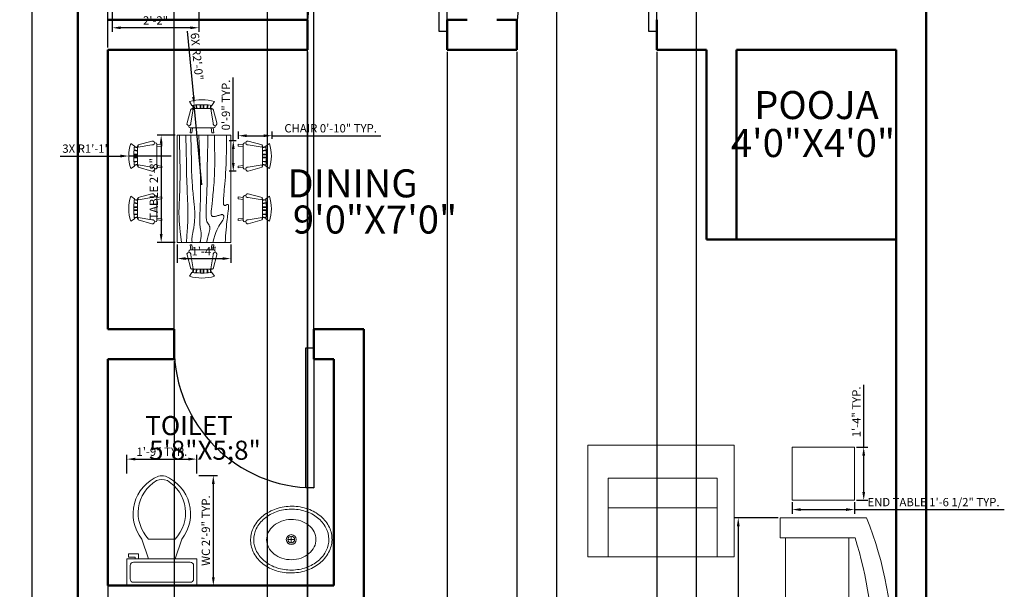
# Model space of a CAD drawing. Units: inches. Extents: x 758743 to 759108, y 3712801 to 3713581.
# Tile 3 of 4: x 758768 to 759064, y 3713244 to 3713415. Entities that reach past the tile are written whole.
import ezdxf

# ---------------------------------------------------------------- set-up
doc = ezdxf.new("R2010")
doc.units = ezdxf.units.IN
for name, color, linetype, lineweight in [('A-ANNO-DIMS', 2, 'Continuous', 18), ('A-AREA-IDEN', 3, 'Continuous', 18), ('A-FLOR-FIXT', 2, 'Continuous', 18), ('A-FURN', 2, 'Continuous', 18), ('DOOR', 4, 'Continuous', 25), ('WALL', 7, 'Continuous', 50)]:
    doc.layers.add(name, color=color, linetype=linetype, lineweight=lineweight)
doc.styles.get("Standard").update_dxf_attribs({"font": 'arial.ttf'})
doc.dimstyles.new('ISO-25', dxfattribs={"dimtxt": 2.5, "dimasz": 2.5, "dimexe": 1.25, "dimexo": 0.625, "dimtad": 1, "dimdec": 0, "dimlunit": 3, "dimtxsty": 'Standard', "dimcen": 2.5, "dimadec": 0, "dimazin": 0, "dimtfac": 1, "dimtdec": 0, "dimtmove": 0, "dimatfit": 3, "dimfxl": 1, "dimarcsym": 0})

# ---------------------------------------------------------------- blocks, each defined once
blk = doc.blocks.new('*U2')
for p, q in [((0, 0), (0, -100)), ((750, 0), (750, -100))]:
    blk.add_line(p, q)
blk.add_lwpolyline([(0, 0), (0, 750), (43.75, 750), (43.75, 0)], close=True)
blk.add_arc((0, 0), 750, 0, 90)
blk = doc.blocks.new('Table - Rectangular Woodgrain 60 x 30 in.')
for p, q in [((0, 0), (0, -30)), ((60, 0), (0, 0)), ((60, -30), (60, 0)), ((0, -30), (60, -30))]:
    blk.add_line(p, q)
for points in [[(0, -2.4), (4.8155, -2.418), (9.0302, -2.4688), (12.709, -2.5477), (15.9167, -2.65), (18.7181, -2.7711), (21.1781, -2.9063), (23.3616, -3.0508), (25.3333, -3.2), (27.1477, -3.3495), (28.8172, -3.4958), (30.3437, -3.636), (31.7291, -3.7667), (32.9756, -3.8849), (34.0849, -3.9875), (35.059, -4.0714), (35.9, -4.1334), (36.6114, -4.1711), (37.2041, -4.1854), (37.6906, -4.1779), (38.0833, -4.15), (38.3948, -4.1034), (38.6375, -4.0396), (38.8239, -3.9602), (38.9666, -3.8667), (39.0764, -3.7608), (39.1573, -3.6448), (39.2116, -3.521), (39.2416, -3.3917), (39.2498, -3.2593), (39.2385, -3.1261), (39.21, -2.9944), (39.1666, -2.8667), (39.111, -2.7447), (39.0468, -2.6281), (38.978, -2.5163), (38.9083, -2.4083), (38.8418, -2.3035), (38.7823, -2.201), (38.7337, -2.1001), (38.7, -2), (38.6844, -1.9003), (38.6875, -1.8021), (38.7094, -1.707), (38.75, -1.6167), (38.8094, -1.5326), (38.8875, -1.4563), (38.9844, -1.3893), (39.1, -1.3333), (39.2351, -1.2896), (39.3937, -1.2583), (39.5804, -1.2396), (39.8, -1.2333), (40.057, -1.2396), (40.3562, -1.2583), (40.7023, -1.2896), (41.1, -1.3333), (41.5547, -1.3895), (42.0755, -1.4573), (42.6721, -1.5361), (43.3542, -1.625), (44.1316, -1.7233), (45.014, -1.8302), (46.0114, -1.9449), (47.1333, -2.0667), (48.3862, -2.1947), (49.7625, -2.3281), (51.2513, -2.4663), (52.8416, -2.6083), (54.5226, -2.7535), (56.2833, -2.9011), (58.1127, -3.0501), (60, -3.2)], [(0, -9.2), (6.5759, -9.0858), (11.9385, -9.0365), (16.2527, -9.0418), (19.6833, -9.0917), (22.3952, -9.1759), (24.5531, -9.2844), (26.322, -9.4069), (27.8666, -9.5333), (29.3241, -9.6553), (30.7203, -9.7719), (32.0532, -9.8837), (33.3208, -9.9917), (34.5213, -10.0965), (35.6526, -10.199), (36.7128, -10.2999), (37.7, -10.4), (38.6129, -10.4996), (39.4531, -10.5969), (40.223, -10.6895), (40.925, -10.775), (41.5613, -10.8512), (42.1344, -10.9156), (42.6465, -10.966), (43.1, -11), (43.4976, -11.0158), (43.8437, -11.0136), (44.143, -10.9942), (44.4, -10.9583), (44.6195, -10.9069), (44.8062, -10.8406), (44.9648, -10.7603), (45.1, -10.6667), (45.2155, -10.5598), (45.3114, -10.4365), (45.3871, -10.2929), (45.4416, -10.125), (45.4743, -9.929), (45.4844, -9.7011), (45.4709, -9.4371), (45.4333, -9.1333), (45.3716, -8.7883), (45.2896, -8.4104), (45.1919, -8.0107), (45.0833, -7.6), (44.9685, -7.1893), (44.8521, -6.7896), (44.7388, -6.4117), (44.6333, -6.0667), (44.54, -5.7628), (44.4614, -5.4979), (44.4001, -5.2675), (44.3583, -5.0667), (44.3384, -4.8909), (44.3427, -4.7354), (44.3736, -4.5956), (44.4333, -4.4667), (44.5236, -4.3453), (44.6427, -4.2333), (44.7884, -4.1339), (44.9583, -4.05), (45.1501, -3.9849), (45.3614, -3.9417), (45.59, -3.9234), (45.8333, -3.9333), (46.0915, -3.9749), (46.3734, -4.0531), (46.6906, -4.1736), (47.0542, -4.3417), (47.4756, -4.5629), (47.9661, -4.8427), (48.5372, -5.1866), (49.2, -5.6), (49.9676, -6.0844), (50.8594, -6.625), (51.8965, -7.2031), (53.1, -7.8), (54.491, -8.3969), (56.0906, -8.975), (57.9199, -9.5156), (60, -10)], [(0, -12.8), (5.1847, -12.9322), (9.6213, -13.0323), (13.3963, -13.1059), (16.5958, -13.1583), (19.3063, -13.1952), (21.614, -13.2219), (23.6054, -13.2439), (25.3666, -13.2667), (26.9728, -13.2947), (28.4531, -13.3281), (29.8256, -13.3663), (31.1083, -13.4083), (32.3191, -13.4535), (33.476, -13.501), (34.597, -13.5501), (35.7, -13.6), (36.7984, -13.6497), (37.8875, -13.6979), (38.9578, -13.743), (40, -13.7833), (41.0047, -13.8174), (41.9625, -13.8438), (42.864, -13.8607), (43.7, -13.8667), (44.4631, -13.8604), (45.1552, -13.8417), (45.7801, -13.8104), (46.3416, -13.7667), (46.8439, -13.7104), (47.2906, -13.6417), (47.6858, -13.5604), (48.0333, -13.4667), (48.3375, -13.3608), (48.6042, -13.2448), (48.8396, -13.121), (49.05, -12.9917), (49.2417, -12.8593), (49.4208, -12.7261), (49.5937, -12.5944), (49.7667, -12.4667), (49.9452, -12.3451), (50.1323, -12.2313), (50.3303, -12.1268), (50.5416, -12.0333), (50.7686, -11.9524), (51.0135, -11.8854), (51.2788, -11.8341), (51.5666, -11.8), (51.8785, -11.7843), (52.2116, -11.7865), (52.562, -11.8059), (52.926, -11.8417), (53.2998, -11.8931), (53.6795, -11.9594), (54.0614, -12.0397), (54.4416, -12.1333), (54.8223, -12.2401), (55.2293, -12.3625), (55.6942, -12.5037), (56.2489, -12.6667), (56.9251, -12.8547), (57.7545, -13.0708), (58.7689, -13.3182), (60, -13.6)], [(0, -18), (5.124, -17.7273), (9.6609, -17.5057), (13.6705, -17.3303), (17.2125, -17.1958), (20.3467, -17.0973), (23.1328, -17.0297), (25.6307, -16.9878), (27.9, -16.9667), (29.9928, -16.9617), (31.9302, -16.9703), (33.7254, -16.9907), (35.3917, -17.0208), (36.9423, -17.0588), (38.3906, -17.1026), (39.7499, -17.1503), (41.0333, -17.2), (42.2519, -17.2496), (43.4073, -17.2969), (44.4986, -17.3395), (45.525, -17.375), (46.4858, -17.4012), (47.3802, -17.4156), (48.2074, -17.416), (48.9667, -17.4), (49.6583, -17.3662), (50.2872, -17.3167), (50.8595, -17.2547), (51.3812, -17.1833), (51.8584, -17.1057), (52.2971, -17.025), (52.7034, -16.9443), (53.0833, -16.8667), (53.443, -16.7951), (53.789, -16.7313), (54.128, -16.6768), (54.4666, -16.6334), (54.8115, -16.6024), (55.1693, -16.5854), (55.5465, -16.5841), (55.95, -16.6), (56.3828, -16.6337), (56.8346, -16.6823), (57.2915, -16.7418), (57.7396, -16.8084), (58.165, -16.878), (58.5539, -16.9469), (58.8924, -17.0111), (59.1666, -17.0667), (59.3679, -17.1107), (59.5078, -17.1438), (59.6032, -17.1675), (59.6708, -17.1833), (59.7275, -17.193), (59.7901, -17.1979), (59.8753, -17.1998), (60, -17.2)], [(0, -22.4), (8.0098, -22.2501), (14.4094, -22.1011), (19.4168, -21.9535), (23.25, -21.8083), (26.1269, -21.6663), (28.2656, -21.5281), (29.884, -21.3947), (31.2, -21.2667), (32.3967, -21.1448), (33.5172, -21.0292), (34.5697, -20.9198), (35.5625, -20.8167), (36.5037, -20.7198), (37.4015, -20.6292), (38.2642, -20.5448), (39.1, -20.4667), (39.9164, -20.3951), (40.7187, -20.3313), (41.5117, -20.2768), (42.3, -20.2333), (43.0883, -20.2024), (43.8812, -20.1854), (44.6836, -20.1841), (45.5, -20.2), (46.3328, -20.234), (47.1747, -20.2844), (48.0163, -20.3488), (48.8479, -20.425), (49.66, -20.5106), (50.4429, -20.6031), (51.1872, -20.7004), (51.8833, -20.8), (52.5246, -20.8999), (53.1166, -20.9995), (53.6681, -21.0983), (54.1875, -21.1958), (54.6834, -21.2919), (55.1646, -21.3859), (55.6394, -21.4777), (56.1167, -21.5667), (56.6028, -21.6515), (57.0961, -21.7266), (57.5929, -21.7852), (58.0896, -21.8208), (58.5823, -21.8268), (59.0674, -21.7964), (59.5412, -21.723), (60, -21.6)], [(0, -25.2), (8.6355, -25.0504), (15.7026, -24.9031), (21.4049, -24.7606), (25.9458, -24.625), (29.529, -24.4988), (32.3578, -24.3844), (34.6359, -24.284), (36.5667, -24.2), (38.3213, -24.1341), (39.9417, -24.0854), (41.437, -24.0523), (42.8167, -24.0333), (44.0901, -24.0268), (45.2667, -24.0313), (46.3557, -24.0451), (47.3667, -24.0667), (48.309, -24.0947), (49.1928, -24.1287), (50.0284, -24.168), (50.826, -24.2125), (51.5959, -24.2617), (52.3483, -24.3151), (53.0935, -24.3725), (53.8417, -24.4334), (54.6009, -24.497), (55.3699, -24.561), (56.1454, -24.6226), (56.9239, -24.6792), (57.7021, -24.7279), (58.4764, -24.7662), (59.2435, -24.7911), (60, -24.8)], [(0, -28.8), (5.6867, -28.6681), (10.45, -28.5698), (14.407, -28.5012), (17.675, -28.4584), (20.3711, -28.4374), (22.6125, -28.4344), (24.5164, -28.4455), (26.2, -28.4667), (27.762, -28.4947), (29.2276, -28.5281), (30.6033, -28.5663), (31.8958, -28.6084), (33.1118, -28.6535), (34.2578, -28.7011), (35.3405, -28.7501), (36.3666, -28.8), (37.3443, -28.8497), (38.288, -28.8974), (39.2137, -28.9412), (40.1375, -28.9792), (41.0753, -29.0093), (42.0432, -29.0297), (43.0572, -29.0384), (44.1333, -29.0333), (45.2936, -29.0114), (46.5843, -28.9641), (48.0579, -28.8816), (49.7666, -28.7542), (51.7629, -28.5721), (54.0989, -28.3255), (56.8272, -28.0048), (60, -27.6)]]:
    blk.add_lwpolyline(points)
blk = doc.blocks.new('Chair - Rocking')
for p, q in [((-9, -7.5), (-12, -18.49999)), ((-8, -4.5), (-10, -1.5)), ((-7, -7.5), (-9, -7.5)), ((-9, -18.49999), (-7, -7.5)), ((-8.23428, -6.99939), (-8.3093, -7.47958)), ((-8.23041, -7), (8.23915, -7)), ((-7.5, -4.5), (-7, -7)), ((-6.5, -7), (-7.02225, -4.43)), ((-4.5, -7), (-4.96674, -4.19951)), ((-4, -7), (-4.40532, -4.16272)), ((-1.5, -4.05012), (-1.5, -7)), ((-1, -7), (-1, -4.05012)), ((1, -7), (1, -4.04655)), ((1.5, -4.05012), (1.5, -7)), ((4, -7), (4.40187, -4.18694)), ((4.5, -7), (4.96761, -4.19437)), ((6.5, -7), (7, -4.4057)), ((7.5, -4.5), (7, -7)), ((7, -7.5), (9, -7.5)), ((9, -18.49999), (7, -7.5)), ((8, -4.5), (10, -1.5)), ((8.31071, -7.48854), (8.23449, -7.00073)), ((9, -7.5), (12, -18.49999)), ((-10.36644, -20.64523), (-10.5, -21.49999)), ((-9, -22.49999), (-9.5, -26.49999)), ((0, -22.49999), (-9.5, -22.49999)), ((-8, -26.49999), (-7.5, -22.49999)), ((0, -22.49999), (9.5, -22.49999)), ((8, -26.49999), (7.5, -22.49999)), ((9, -22.49999), (9.5, -26.49999)), ((10.5, -21.49999), (10.3575, -20.58798)), ((-9.5, -26.49999), (-8, -26.49999)), ((9.5, -26.49999), (8, -26.49999))]:
    blk.add_line(p, q)
for centre, radius, start, end in [((0, -34.08333), 34.08333, 72.93847, 107.0615), ((0, -68.25004), 64.25, 93.92211, 97.15267), ((0, -68.25004), 64.25, 82.84733, 93.92211), ((-10.5, -18.99999), 1.58114, 161.5651, 18.43495), ((-9.5, -21.49999), 1, 180, 270), ((10.5, -18.99999), 1.58114, 161.5651, 18.43495), ((9.5, -21.49999), 1, 270, 0)]:
    blk.add_arc(centre, radius, start, end)
blk = doc.blocks.new('Toilet - top')
for p, q in [((9.5, -6), (9.5, -2)), ((-10, -8.5), (-8, -8.5)), ((-10, -9.5), (-10, -8.5)), ((-8, -8.5), (-8, -8)), ((-7, -8), (-7, -9.5)), ((-4, -8), (-6, -14)), ((4, -8), (6, -14)), ((-7, -9.5), (-10, -9.5)), ((4, -14), (-4, -14))]:
    blk.add_line(p, q)
blk.add_lwpolyline([(10.5, -8), (10.5, 0), (-10.5, 0), (-10.5, -8)], close=True)
for points in [[(-9.5, -2), (-9.5, -6)], [(8.5, -1), (-8.5, -1)], [(-8.5, -7), (8.5, -7)]]:
    blk.add_lwpolyline(points)
for centre, radius, start, end in [((-8.62, -1.88), 0.884, 81.8699, 188.1301), ((8.62, -1.88), 0.884, 351.8699, 98.1301), ((-8.62, -6.12), 0.884, 171.8699, 278.1301), ((8.62, -6.12), 0.884, 261.8699, 8.1301), ((3.52, -21.58), 12.17, 141.4691, 247.9714), ((4.2, -21.82), 11.33, 136.3677, 238.9468), ((-3.52, -21.58), 12.17, 292.0284, 38.5307), ((-4.2, -21.82), 11.33, 301.053, 43.6321), ((0, -27.88), 4, 245.7318, 294.2682), ((0, -29), 4, 254.8605, 285.1395)]:
    blk.add_arc(centre, radius, start, end)
blk = doc.blocks.new('Sink - Oval top')
for p, q in [((-1, 0), (1, 0)), ((0, 1), (0, -1))]:
    blk.add_line(p, q)
for points in [[(-12.23, 0.39, 0.117634), (-11.46, -3.36, 0.104469), (-8.88, -6.8, 0.090016), (-5.08, -9.07, 0.08192), (-0.32, -10.02, 0.08192), (4.49, -9.38, 0.090016), (8.42, -7.36, 0.104469), (11.22, -4.09, 0.117634), (12.23, -0.39, 0.117634), (11.46, 3.36, 0.104469), (8.88, 6.8, 0.090016), (5.08, 9.07, 0.08192), (0.32, 10.02, 0.08192), (-4.49, 9.38, 0.090016), (-8.42, 7.36, 0.104469), (-11.22, 4.09, 0.117634)], [(-11.29, 0.16, 0.118622), (-10.52, -3.25, 0.104678), (-8.07, -6.36, 0.089562), (-4.54, -8.37, 0.081185), (-0.13, -9.15, 0.081185), (4.3, -8.49, 0.089562), (7.89, -6.58, 0.104678), (10.42, -3.55, 0.118622), (11.29, -0.16, 0.118622), (10.52, 3.25, 0.104678), (8.07, 6.36, 0.089562), (4.54, 8.37, 0.081185), (0.13, 9.15, 0.081185), (-4.3, 8.49, 0.089562), (-7.89, 6.58, 0.104678), (-10.42, 3.55, 0.118622)], [(-7.42, 0.08, 0.118283), (-6.91, -2.17, 0.104607), (-5.29, -4.21, 0.089718), (-2.97, -5.53, 0.081436), (-0.07, -6.04, 0.081436), (2.84, -5.59, 0.089718), (5.2, -4.33, 0.104607), (6.86, -2.32, 0.118283), (7.42, -0.08, 0.118283), (6.91, 2.17, 0.104607), (5.29, 4.21, 0.089718), (2.97, 5.53, 0.081436), (0.07, 6.04, 0.081436), (-2.84, 5.59, 0.089718), (-5.2, 4.33, 0.104607), (-6.86, 2.32, 0.118283)]]:
    blk.add_lwpolyline(points, format="xyb", close=True)
for radius in [1.5, 1]:
    blk.add_circle((0, 0), radius)
blk = doc.blocks.new('Sofa - Roundback 7 ft.')
for p, q in [((-12.00002, -32.4421), (-12.00003, -6.5971)), ((11.99997, -32.4421), (11.99998, -6.5971)), ((-36.000027, -34), (-36.000027, -11.4696)), ((35.99998, -34), (35.99998, -11.4696)), ((-35.999844, -13.3819), (35.9998, -13.3819)), ((-36.000027, -32.4421), (35.99998, -32.4421))]:
    blk.add_line(p, q)
for points in [[(-36.000027, -34), (-42.000027, -34), (-42.000027, -8)], [(41.99998, -8), (41.99998, -34), (35.99998, -34)]]:
    blk.add_lwpolyline(points)
for centre, radius, start, end in [((0, -114.25), 114.25, 68.43141, 111.5686), ((-0.00001, -127.1968), 121.1968, 72.72033, 107.2797)]:
    blk.add_arc(centre, radius, start, end)
blk = doc.blocks.new('*D13')
at = {"layer": 'A-ANNO-DIMS', "color": 0, "lineweight": -2, "transparency": 16777216}
for p, q in [((758785.26, 3713540.49), (758770.79, 3713540.49)), ((758772.04, 3713537.99), (758772.04, 3712841.99)), ((758785.26, 3712839.49), (758770.79, 3712839.49))]:
    blk.add_line(p, q, dxfattribs=at)
at = {"layer": 'A-ANNO-DIMS', "color": 0, "transparency": 16777216}
for points in [[(758771.62, 3713537.99), (758772.46, 3713537.99), (758772.04, 3713540.49)], [(758771.62, 3712841.99), (758772.46, 3712841.99), (758772.04, 3712839.49)]]:
    blk.add_solid(points, dxfattribs=at)
at = {"layer": 'Defpoints', "color": 0, "transparency": 16777216}
for p in [(758785.89, 3713540.49), (758772.04, 3712839.49), (758785.89, 3712839.49)]:
    blk.add_point(p, dxfattribs=at)
at = {"layer": 'A-ANNO-DIMS', "color": 0, "transparency": 16777216, "insert": (758770.14, 3713189.99), "char_height": 2.5, "attachment_point": 5, "rotation": 90}
blk.add_mtext('58\'-5"', dxfattribs=at)
blk = doc.blocks.new('END-TABLE')
blk.add_lwpolyline([(0, 15.93), (18.69, 15.93), (18.69, 0), (0, 0)], close=True)
blk = doc.blocks.new('*D18')
at = {"layer": 'A-ANNO-DIMS', "color": 0, "lineweight": -2, "transparency": 16777216}
for p, q in [((758834.15, 3713379.74), (758834.15, 3713381.89)), ((758836.65, 3713380.64), (758841.77, 3713380.64)), ((758844.27, 3713379.74), (758844.27, 3713381.89)), ((758844.27, 3713380.64), (758877.01, 3713380.64))]:
    blk.add_line(p, q, dxfattribs=at)
at = {"layer": 'A-ANNO-DIMS', "color": 0, "transparency": 16777216}
for points in [[(758836.65, 3713381.05), (758836.65, 3713380.22), (758834.15, 3713380.64)], [(758841.77, 3713381.05), (758841.77, 3713380.22), (758844.27, 3713380.64)]]:
    blk.add_solid(points, dxfattribs=at)
at = {"layer": 'Defpoints', "color": 0, "transparency": 16777216}
for p in [(758844.27, 3713380.64), (758834.15, 3713379.12), (758844.27, 3713379.12)]:
    blk.add_point(p, dxfattribs=at)
at = {"layer": 'A-ANNO-DIMS', "color": 0, "transparency": 16777216, "insert": (758861.89, 3713382.55), "char_height": 2.5, "attachment_point": 5}
blk.add_mtext('CHAIR 0\'-10" TYP.', dxfattribs=at)
blk = doc.blocks.new('*D19')
at = {"layer": 'A-ANNO-DIMS', "color": 0, "lineweight": -2, "transparency": 16777216}
for p, q in [((758832.63, 3713379.12), (758832.63, 3713398.11)), ((758833.52, 3713379.12), (758831.38, 3713379.12)), ((758832.63, 3713372.46), (758832.63, 3713376.62)), ((758833.52, 3713369.96), (758831.38, 3713369.96))]:
    blk.add_line(p, q, dxfattribs=at)
at = {"layer": 'A-ANNO-DIMS', "color": 0, "transparency": 16777216}
for points in [[(758832.21, 3713376.62), (758833.05, 3713376.62), (758832.63, 3713379.12)], [(758832.21, 3713372.46), (758833.05, 3713372.46), (758832.63, 3713369.96)]]:
    blk.add_solid(points, dxfattribs=at)
at = {"layer": 'Defpoints', "color": 0, "transparency": 16777216}
for p in [(758832.63, 3713379.12), (758834.15, 3713379.12), (758834.15, 3713369.96)]:
    blk.add_point(p, dxfattribs=at)
at = {"layer": 'A-ANNO-DIMS', "color": 0, "transparency": 16777216, "insert": (758830.73, 3713389.86), "char_height": 2.5, "attachment_point": 5, "rotation": 90}
blk.add_mtext('0\'-9" TYP.', dxfattribs=at)
blk = doc.blocks.new('*D20')
at = {"layer": 'A-ANNO-DIMS', "color": 0, "lineweight": -2, "transparency": 16777216}
for p, q in [((758815.16, 3713380.76), (758809.71, 3713380.76)), ((758810.96, 3713378.26), (758810.96, 3713351.07)), ((758815.16, 3713348.57), (758809.71, 3713348.57))]:
    blk.add_line(p, q, dxfattribs=at)
at = {"layer": 'A-ANNO-DIMS', "color": 0, "transparency": 16777216}
for points in [[(758810.54, 3713378.26), (758811.38, 3713378.26), (758810.96, 3713380.76)], [(758810.54, 3713351.07), (758811.38, 3713351.07), (758810.96, 3713348.57)]]:
    blk.add_solid(points, dxfattribs=at)
at = {"layer": 'Defpoints', "color": 0, "transparency": 16777216}
for p in [(758815.79, 3713380.76), (758810.96, 3713348.57), (758815.79, 3713348.57)]:
    blk.add_point(p, dxfattribs=at)
at = {"layer": 'A-ANNO-DIMS', "color": 0, "transparency": 16777216, "insert": (758809.06, 3713364.67), "char_height": 2.5, "attachment_point": 5, "rotation": 90}
blk.add_mtext('TABLE 2\'-8"', dxfattribs=at)
blk = doc.blocks.new('*D21')
at = {"layer": 'A-ANNO-DIMS', "color": 0, "lineweight": -2, "transparency": 16777216}
for p, q in [((758815.79, 3713347.94), (758815.79, 3713342.49)), ((758831.89, 3713347.94), (758831.89, 3713342.49)), ((758818.29, 3713343.74), (758829.39, 3713343.74))]:
    blk.add_line(p, q, dxfattribs=at)
at = {"layer": 'A-ANNO-DIMS', "color": 0, "transparency": 16777216}
for points in [[(758818.29, 3713344.15), (758818.29, 3713343.32), (758815.79, 3713343.74)], [(758829.39, 3713344.15), (758829.39, 3713343.32), (758831.89, 3713343.74)]]:
    blk.add_solid(points, dxfattribs=at)
at = {"layer": 'Defpoints', "color": 0, "transparency": 16777216}
for p in [(758815.79, 3713348.57), (758831.89, 3713348.57), (758831.89, 3713343.74)]:
    blk.add_point(p, dxfattribs=at)
at = {"layer": 'A-ANNO-DIMS', "color": 0, "transparency": 16777216, "insert": (758823.84, 3713345.62), "char_height": 2.5, "attachment_point": 5}
blk.add_mtext('1\'-4"', dxfattribs=at)
blk = doc.blocks.new('*D22')
at = {"layer": 'A-ANNO-DIMS', "color": 0, "lineweight": -2, "transparency": 16777216}
for p, q in [((758822.3, 3713278.54), (758827.88, 3713278.54)), ((758826.63, 3713276.04), (758826.63, 3713247.99)), ((758822.3, 3713245.49), (758827.88, 3713245.49))]:
    blk.add_line(p, q, dxfattribs=at)
at = {"layer": 'A-ANNO-DIMS', "color": 0, "transparency": 16777216}
for points in [[(758826.21, 3713276.04), (758827.05, 3713276.04), (758826.63, 3713278.54)], [(758826.21, 3713247.99), (758827.05, 3713247.99), (758826.63, 3713245.49)]]:
    blk.add_solid(points, dxfattribs=at)
at = {"layer": 'Defpoints', "color": 0, "transparency": 16777216}
for p in [(758821.67, 3713278.54), (758821.67, 3713245.49), (758826.63, 3713245.49)]:
    blk.add_point(p, dxfattribs=at)
at = {"layer": 'A-ANNO-DIMS', "color": 0, "transparency": 16777216, "insert": (758824.71, 3713262.01), "char_height": 2.5, "attachment_point": 5, "rotation": 90}
blk.add_mtext('WC 2\'-9" TYP.', dxfattribs=at)
blk = doc.blocks.new('*D23')
at = {"layer": 'A-ANNO-DIMS', "color": 0, "lineweight": -2, "transparency": 16777216}
for p, q in [((758800.67, 3713279.16), (758800.67, 3713284.74)), ((758803.17, 3713283.49), (758819.17, 3713283.49)), ((758821.67, 3713279.16), (758821.67, 3713284.74))]:
    blk.add_line(p, q, dxfattribs=at)
at = {"layer": 'A-ANNO-DIMS', "color": 0, "transparency": 16777216}
for points in [[(758803.17, 3713283.91), (758803.17, 3713283.08), (758800.67, 3713283.49)], [(758819.17, 3713283.91), (758819.17, 3713283.08), (758821.67, 3713283.49)]]:
    blk.add_solid(points, dxfattribs=at)
at = {"layer": 'Defpoints', "color": 0, "transparency": 16777216}
for p in [(758821.67, 3713283.49), (758800.67, 3713278.54), (758821.67, 3713278.54)]:
    blk.add_point(p, dxfattribs=at)
at = {"layer": 'A-ANNO-DIMS', "color": 0, "transparency": 16777216, "insert": (758811.17, 3713285.4), "char_height": 2.5, "attachment_point": 5}
blk.add_mtext('1\'-9" TYP.', dxfattribs=at)
blk = doc.blocks.new('*D34')
at = {"layer": 'A-ANNO-DIMS', "color": 0, "lineweight": -2, "transparency": 16777216}
for p, q in [((759000.62, 3713270.51), (759000.62, 3713267.08)), ((759003.12, 3713268.33), (759016.81, 3713268.33)), ((759019.31, 3713270.51), (759019.31, 3713267.08)), ((759019.31, 3713268.33), (759064.37, 3713268.33))]:
    blk.add_line(p, q, dxfattribs=at)
at = {"layer": 'A-ANNO-DIMS', "color": 0, "transparency": 16777216}
for points in [[(759003.12, 3713268.75), (759003.12, 3713267.91), (759000.62, 3713268.33)], [(759016.81, 3713268.75), (759016.81, 3713267.91), (759019.31, 3713268.33)]]:
    blk.add_solid(points, dxfattribs=at)
at = {"layer": 'Defpoints', "color": 0, "transparency": 16777216}
for p in [(759000.62, 3713271.13), (759019.31, 3713271.13), (759019.31, 3713268.33)]:
    blk.add_point(p, dxfattribs=at)
at = {"layer": 'A-ANNO-DIMS', "color": 0, "transparency": 16777216, "insert": (759043.09, 3713270.25), "char_height": 2.5, "attachment_point": 5}
blk.add_mtext('END TABLE 1\'-6 1/2" TYP.', dxfattribs=at)
blk = doc.blocks.new('*D35')
at = {"layer": 'A-ANNO-DIMS', "color": 0, "lineweight": -2, "transparency": 16777216}
for p, q in [((759022.11, 3713287.07), (759022.11, 3713305.82)), ((759019.93, 3713287.07), (759023.36, 3713287.07)), ((759022.11, 3713273.63), (759022.11, 3713284.57)), ((759019.93, 3713271.13), (759023.36, 3713271.13))]:
    blk.add_line(p, q, dxfattribs=at)
at = {"layer": 'A-ANNO-DIMS', "color": 0, "transparency": 16777216}
for points in [[(759021.69, 3713284.57), (759022.53, 3713284.57), (759022.11, 3713287.07)], [(759021.69, 3713273.63), (759022.53, 3713273.63), (759022.11, 3713271.13)]]:
    blk.add_solid(points, dxfattribs=at)
at = {"layer": 'Defpoints', "color": 0, "transparency": 16777216}
for p in [(759019.31, 3713287.07), (759022.11, 3713287.07), (759019.31, 3713271.13)]:
    blk.add_point(p, dxfattribs=at)
at = {"layer": 'A-ANNO-DIMS', "color": 0, "transparency": 16777216, "insert": (759020.23, 3713297.69), "char_height": 2.5, "attachment_point": 5, "rotation": 90}
blk.add_mtext('1\'-4" TYP.', dxfattribs=at)
blk = doc.blocks.new('*D39')
at = {"layer": 'A-ANNO-DIMS', "color": 0, "lineweight": -2, "transparency": 16777216}
for p, q in [((758796.27, 3713417.84), (758796.27, 3713411.82)), ((758822.27, 3713417.84), (758822.27, 3713411.82)), ((758819.77, 3713413.07), (758798.77, 3713413.07))]:
    blk.add_line(p, q, dxfattribs=at)
at = {"layer": 'A-ANNO-DIMS', "color": 0, "transparency": 16777216}
for points in [[(758798.77, 3713413.48), (758798.77, 3713412.65), (758796.27, 3713413.07)], [(758819.77, 3713413.48), (758819.77, 3713412.65), (758822.27, 3713413.07)]]:
    blk.add_solid(points, dxfattribs=at)
at = {"layer": 'Defpoints', "color": 0, "transparency": 16777216}
for p in [(758796.27, 3713418.47), (758822.27, 3713418.47), (758796.27, 3713413.07)]:
    blk.add_point(p, dxfattribs=at)
at = {"layer": 'A-ANNO-DIMS', "color": 0, "transparency": 16777216, "insert": (758809.27, 3713414.95), "char_height": 2.5, "attachment_point": 5}
blk.add_mtext('2\'-2"', dxfattribs=at)
blk = doc.blocks.new('*D40')
at = {"layer": 'A-ANNO-DIMS', "color": 0, "lineweight": -2, "transparency": 16777216}
for p, q in [((758996.38, 3713265.84), (758983.15, 3713265.84)), ((758984.4, 3713263.34), (758984.4, 3713184.34)), ((758996.38, 3713181.84), (758983.15, 3713181.84))]:
    blk.add_line(p, q, dxfattribs=at)
at = {"layer": 'A-ANNO-DIMS', "color": 0, "transparency": 16777216}
for points in [[(758983.99, 3713263.34), (758984.82, 3713263.34), (758984.4, 3713265.84)], [(758983.99, 3713184.34), (758984.82, 3713184.34), (758984.4, 3713181.84)]]:
    blk.add_solid(points, dxfattribs=at)
at = {"layer": 'Defpoints', "color": 0, "transparency": 16777216}
for p in [(758997, 3713265.84), (758984.4, 3713181.84), (758997, 3713181.84)]:
    blk.add_point(p, dxfattribs=at)
at = {"layer": 'A-ANNO-DIMS', "color": 0, "transparency": 16777216, "insert": (758982.48, 3713223.84), "char_height": 2.5, "attachment_point": 5, "rotation": 90}
blk.add_mtext('SOFA 7\'-0"', dxfattribs=at)
blk = doc.blocks.new('*D46')
at = {"layer": 'A-ANNO-DIMS', "color": 0, "lineweight": -2, "transparency": 16777216}
for p, q in [((758842.89, 3712849.12), (758842.89, 3713578.64)), ((758854.89, 3712849.12), (758854.89, 3713578.64)), ((758845.39, 3713577.39), (758852.39, 3713577.39))]:
    blk.add_line(p, q, dxfattribs=at)
at = {"layer": 'A-ANNO-DIMS', "color": 0, "transparency": 16777216}
for points in [[(758845.39, 3713577.81), (758845.39, 3713576.97), (758842.89, 3713577.39)], [(758852.39, 3713577.81), (758852.39, 3713576.97), (758854.89, 3713577.39)]]:
    blk.add_solid(points, dxfattribs=at)
at = {"layer": 'Defpoints', "color": 0, "transparency": 16777216}
for p in [(758854.89, 3713577.39), (758842.89, 3712848.49), (758854.89, 3712848.49)]:
    blk.add_point(p, dxfattribs=at)
at = {"layer": 'A-ANNO-DIMS', "color": 0, "transparency": 16777216, "insert": (758848.89, 3713579.29), "char_height": 2.5, "attachment_point": 5}
blk.add_mtext('1\'-0"', dxfattribs=at)
blk = doc.blocks.new('*D49')
at = {"layer": 'A-ANNO-DIMS', "color": 0, "lineweight": -2, "transparency": 16777216}
for p, q in [((758929.89, 3713089.12), (758929.89, 3713578.64)), ((758971.89, 3713089.12), (758971.89, 3713578.64)), ((758932.39, 3713577.39), (758969.39, 3713577.39))]:
    blk.add_line(p, q, dxfattribs=at)
at = {"layer": 'A-ANNO-DIMS', "color": 0, "transparency": 16777216}
for points in [[(758932.39, 3713577.81), (758932.39, 3713576.97), (758929.89, 3713577.39)], [(758969.39, 3713577.81), (758969.39, 3713576.97), (758971.89, 3713577.39)]]:
    blk.add_solid(points, dxfattribs=at)
at = {"layer": 'Defpoints', "color": 0, "transparency": 16777216}
for p in [(758971.89, 3713577.39), (758929.89, 3713088.49), (758971.89, 3713088.49)]:
    blk.add_point(p, dxfattribs=at)
at = {"layer": 'A-ANNO-DIMS', "color": 0, "transparency": 16777216, "insert": (758950.89, 3713579.29), "char_height": 2.5, "attachment_point": 5}
blk.add_mtext('3\'-6"', dxfattribs=at)
blk = doc.blocks.new('*D50')
at = {"layer": 'A-ANNO-DIMS', "color": 0, "lineweight": -2, "transparency": 16777216}
for p, q in [((758794.89, 3713312.87), (758794.89, 3712801.34)), ((758814.89, 3713312.87), (758814.89, 3712801.34)), ((758797.39, 3712802.59), (758812.39, 3712802.59))]:
    blk.add_line(p, q, dxfattribs=at)
at = {"layer": 'A-ANNO-DIMS', "color": 0, "transparency": 16777216}
for points in [[(758797.39, 3712803.01), (758797.39, 3712802.17), (758794.89, 3712802.59)], [(758812.39, 3712803.01), (758812.39, 3712802.17), (758814.89, 3712802.59)]]:
    blk.add_solid(points, dxfattribs=at)
at = {"layer": 'Defpoints', "color": 0, "transparency": 16777216}
for p in [(758794.89, 3713313.49), (758814.89, 3713313.49), (758814.89, 3712802.59)]:
    blk.add_point(p, dxfattribs=at)
at = {"layer": 'A-ANNO-DIMS', "color": 0, "transparency": 16777216, "insert": (758804.89, 3712804.49), "char_height": 2.5, "attachment_point": 5}
blk.add_mtext('1\'-8"', dxfattribs=at)
blk = doc.blocks.new('*D51')
at = {"layer": 'A-ANNO-DIMS', "color": 0, "lineweight": -2, "transparency": 16777216}
for p, q in [((758814.89, 3713314.12), (758814.89, 3713578.64)), ((758856.89, 3713314.12), (758856.89, 3713578.64)), ((758817.39, 3713577.39), (758854.39, 3713577.39))]:
    blk.add_line(p, q, dxfattribs=at)
at = {"layer": 'A-ANNO-DIMS', "color": 0, "transparency": 16777216}
for points in [[(758817.39, 3713577.81), (758817.39, 3713576.97), (758814.89, 3713577.39)], [(758854.39, 3713577.81), (758854.39, 3713576.97), (758856.89, 3713577.39)]]:
    blk.add_solid(points, dxfattribs=at)
at = {"layer": 'Defpoints', "color": 0, "transparency": 16777216}
for p in [(758856.89, 3713577.39), (758814.89, 3713313.49), (758856.89, 3713313.49)]:
    blk.add_point(p, dxfattribs=at)
at = {"layer": 'A-ANNO-DIMS', "color": 0, "transparency": 16777216, "insert": (758835.89, 3713579.29), "char_height": 2.5, "attachment_point": 5}
blk.add_mtext('3\'-6"', dxfattribs=at)
blk = doc.blocks.new('*D53')
at = {"layer": 'A-ANNO-DIMS', "color": 0, "lineweight": -2, "transparency": 16777216}
for p, q in [((758794.89, 3713407.12), (758794.89, 3713578.64)), ((758854.89, 3713407.12), (758854.89, 3713578.64)), ((758797.39, 3713577.39), (758852.39, 3713577.39))]:
    blk.add_line(p, q, dxfattribs=at)
at = {"layer": 'A-ANNO-DIMS', "color": 0, "transparency": 16777216}
for points in [[(758797.39, 3713577.81), (758797.39, 3713576.97), (758794.89, 3713577.39)], [(758852.39, 3713577.81), (758852.39, 3713576.97), (758854.89, 3713577.39)]]:
    blk.add_solid(points, dxfattribs=at)
at = {"layer": 'Defpoints', "color": 0, "transparency": 16777216}
for p in [(758854.89, 3713577.39), (758794.89, 3713406.49), (758854.89, 3713406.49)]:
    blk.add_point(p, dxfattribs=at)
at = {"layer": 'A-ANNO-DIMS', "color": 0, "transparency": 16777216, "insert": (758824.89, 3713579.29), "char_height": 2.5, "attachment_point": 5}
blk.add_mtext('5\'-0"', dxfattribs=at)
blk = doc.blocks.new('*D54')
at = {"layer": 'A-ANNO-DIMS', "color": 0, "lineweight": -2, "transparency": 16777216}
for p, q in [((758854.89, 3713405.87), (758854.89, 3712801.34)), ((758896.89, 3713405.87), (758896.89, 3712801.34)), ((758857.39, 3712802.59), (758894.39, 3712802.59))]:
    blk.add_line(p, q, dxfattribs=at)
at = {"layer": 'A-ANNO-DIMS', "color": 0, "transparency": 16777216}
for points in [[(758857.39, 3712803.01), (758857.39, 3712802.17), (758854.89, 3712802.59)], [(758894.39, 3712803.01), (758894.39, 3712802.17), (758896.89, 3712802.59)]]:
    blk.add_solid(points, dxfattribs=at)
at = {"layer": 'Defpoints', "color": 0, "transparency": 16777216}
for p in [(758854.89, 3713406.49), (758896.89, 3713406.49), (758896.89, 3712802.59)]:
    blk.add_point(p, dxfattribs=at)
at = {"layer": 'A-ANNO-DIMS', "color": 0, "transparency": 16777216, "insert": (758875.89, 3712804.49), "char_height": 2.5, "attachment_point": 5}
blk.add_mtext('3\'-6"', dxfattribs=at)
blk = doc.blocks.new('*D59')
at = {"layer": 'A-ANNO-DIMS', "color": 0, "lineweight": -2, "transparency": 16777216}
for p, q in [((758917.89, 3713405.87), (758917.89, 3712801.34)), ((758959.89, 3713405.87), (758959.89, 3712801.34)), ((758920.39, 3712802.59), (758957.39, 3712802.59))]:
    blk.add_line(p, q, dxfattribs=at)
at = {"layer": 'A-ANNO-DIMS', "color": 0, "transparency": 16777216}
for points in [[(758920.39, 3712803.01), (758920.39, 3712802.17), (758917.89, 3712802.59)], [(758957.39, 3712803.01), (758957.39, 3712802.17), (758959.89, 3712802.59)]]:
    blk.add_solid(points, dxfattribs=at)
at = {"layer": 'Defpoints', "color": 0, "transparency": 16777216}
for p in [(758917.89, 3713406.49), (758959.89, 3713406.49), (758959.89, 3712802.59)]:
    blk.add_point(p, dxfattribs=at)
at = {"layer": 'A-ANNO-DIMS', "color": 0, "transparency": 16777216, "insert": (758938.89, 3712804.49), "char_height": 2.5, "attachment_point": 5}
blk.add_mtext('3\'-6"', dxfattribs=at)
blk = doc.blocks.new('*D63')
at = {"layer": 'A-ANNO-DIMS', "color": 0, "lineweight": -2, "transparency": 16777216}
for p, q in [((758818.75, 3713412.02), (758820.66, 3713392.33)), ((758823.22, 3713365.86), (758820.9, 3713389.84))]:
    blk.add_line(p, q, dxfattribs=at)
at = {"layer": 'A-ANNO-DIMS', "color": 0, "transparency": 16777216}
blk.add_solid([(758821.07, 3713392.37), (758820.24, 3713392.29), (758820.9, 3713389.84)], dxfattribs=at)
at = {"layer": 'Defpoints', "color": 0, "transparency": 16777216}
for p in [(758820.9, 3713389.84), (758823.22, 3713365.86)]:
    blk.add_point(p, dxfattribs=at)
at = {"layer": 'A-ANNO-DIMS', "color": 0, "transparency": 16777216, "insert": (758821.39, 3713404.41), "char_height": 2.5, "attachment_point": 5, "rotation": 275.5373}
blk.add_mtext('6X R2\'-0"', dxfattribs=at)
blk = doc.blocks.new('*D64')
at = {"layer": 'A-ANNO-DIMS', "color": 0, "lineweight": -2, "transparency": 16777216}
for p, q in [((758780.57, 3713374.54), (758798.73, 3713374.54)), ((758814.01, 3713374.54), (758801.23, 3713374.54))]:
    blk.add_line(p, q, dxfattribs=at)
at = {"layer": 'A-ANNO-DIMS', "color": 0, "transparency": 16777216}
blk.add_solid([(758798.73, 3713374.95), (758798.73, 3713374.12), (758801.23, 3713374.54)], dxfattribs=at)
at = {"layer": 'Defpoints', "color": 0, "transparency": 16777216}
for p in [(758801.23, 3713374.54), (758814.01, 3713374.54)]:
    blk.add_point(p, dxfattribs=at)
at = {"layer": 'A-ANNO-DIMS', "color": 0, "transparency": 16777216, "insert": (758788.4, 3713376.44), "char_height": 2.5, "attachment_point": 5, "rotation": 0.0002}
blk.add_mtext('3X R1\'-1"', dxfattribs=at)

msp = doc.modelspace()

# ---------------------------------------------------------------- linework, layer by layer
at = {"layer": 'A-FURN'}
for p, q in [((758978.09, 3713277.77), (758945.31, 3713277.77)), ((758945.31, 3713277.77), (758945.31, 3713254.15)), ((758978.09, 3713254.15), (758978.09, 3713277.77)), ((758945.31, 3713268.89), (758978.09, 3713268.89))]:
    msp.add_line(p, q, dxfattribs=at)
msp.add_lwpolyline([(758939.15, 3713287.67), (758983.13, 3713287.67), (758983.13, 3713254.15), (758939.15, 3713254.15)], close=True, dxfattribs=at)
at = {"layer": 'WALL'}
for p, q in [((758785.89, 3713540.49), (758785.89, 3712839.49)), ((759040.89, 3713540.49), (759040.89, 3712839.49)), ((758794.89, 3713415.49), (758854.89, 3713415.49)), ((758854.89, 3713415.49), (758854.89, 3713406.49)), ((758896.89, 3713415.49), (758896.89, 3713406.49)), ((758896.89, 3713415.49), (758902.89, 3713415.49)), ((758911.89, 3713415.49), (758917.89, 3713415.49)), ((758917.89, 3713415.49), (758917.89, 3713406.49)), ((758959.89, 3713415.49), (758959.89, 3713406.49)), ((758794.89, 3713406.49), (758854.89, 3713406.49)), ((758794.89, 3713406.49), (758794.89, 3713322.49)), ((758896.89, 3713406.49), (758917.89, 3713406.49)), ((758959.89, 3713406.49), (758974.89, 3713406.49)), ((758974.89, 3713406.49), (758974.89, 3713349.49)), ((758983.89, 3713406.49), (758983.89, 3713349.49)), ((758983.89, 3713406.49), (759031.89, 3713406.49)), ((759031.89, 3713406.49), (759031.89, 3712848.49)), ((758974.89, 3713349.49), (759031.89, 3713349.49)), ((758794.89, 3713322.49), (758814.89, 3713322.49)), ((758814.89, 3713313.49), (758814.89, 3713322.49)), ((758856.89, 3713313.49), (758856.89, 3713322.49)), ((758856.89, 3713322.49), (758871.89, 3713322.49)), ((758871.89, 3713322.49), (758871.89, 3713159.49)), ((758794.89, 3713313.49), (758814.89, 3713313.49)), ((758794.89, 3713313.49), (758794.89, 3713245.49)), ((758856.89, 3713313.49), (758862.89, 3713313.49)), ((758862.89, 3713313.49), (758862.89, 3713245.49)), ((758794.89, 3713245.49), (758862.89, 3713245.49))]:
    msp.add_line(p, q, dxfattribs=at)

# ---------------------------------------------------------------- block references
at = {"layer": 'A-FLOR-FIXT', "xscale": -1, "rotation": 180}
for name, p in [('Toilet - top', (758811.17, 3713245.49)), ('Sink - Oval top', (758850.07, 3713259.31))]:
    msp.add_blockref(name, p, dxfattribs=at)
at = {"layer": 'A-FURN', "xscale": 0.3749312349582522, "yscale": 0.3749312349582522, "zscale": 0.3749312349582522}
msp.add_blockref('Chair - Rocking', (758823.22, 3713391.45), dxfattribs=at)
at = {"layer": 'A-FURN'}
for name, p, xscale, yscale, zscale, rotation in [('Table - Rectangular Woodgrain 60 x 30 in.', (758831.89, 3713380.76), 0.5366550353784367, 0.5366550353784367, 0.5366550353784367, 270), ('Chair - Rocking', (758801.23, 3713374.54), 0.3749312349582522, 0.3749312349582522, 0.3749312349582522, 90.00000000000003), ('Chair - Rocking', (758844.08, 3713374.54), -0.3749312349582522, 0.3749312349582522, 0.3749312349582522, 270), ('Chair - Rocking', (758801.23, 3713358.71), 0.3749312349582522, 0.3749312349582522, 0.3749312349582522, 90.00000000000003), ('Chair - Rocking', (758844.08, 3713358.71), -0.3749312349582522, 0.3749312349582522, 0.3749312349582522, 270), ('Chair - Rocking', (758823.22, 3713337.88), -0.3749312349582522, 0.3749312349582522, 0.3749312349582522, 180)]:
    msp.add_blockref(name, p, dxfattribs=dict(at, xscale=xscale, yscale=yscale, zscale=zscale, rotation=rotation))
msp.add_blockref('END-TABLE', (759000.62, 3713271.13), dxfattribs=at)
at = {"layer": 'A-FURN', "rotation": 270}
msp.add_blockref('Sofa - Roundback 7 ft.', (759031, 3713223.84), dxfattribs=at)
at = {"layer": 'DOOR', "xscale": -0.0559999999999739, "yscale": 0.0559999999999739, "zscale": 0.0559999999999739}
for p in [(758896.89, 3713412.09), (758959.89, 3713412.09)]:
    msp.add_blockref('*U2', p, dxfattribs=at)
at = {"layer": 'DOOR', "xscale": 0.0559999999999739, "yscale": 0.0559999999999739, "zscale": 0.0559999999999739, "rotation": 180}
msp.add_blockref('*U2', (758856.89, 3713316.89), dxfattribs=at)

# ---------------------------------------------------------------- texts
at = {"layer": 'A-AREA-IDEN'}
for s, height, p in [('POOJA', 8.421, (758989.19, 3713385.64)), ('4\'0"X4\'0"', 8.421, (758982.17, 3713374.23)), ('DINING', 8.421, (758848.88, 3713362.12)), ('9\'0"X7\'0"', 8.421, (758850.54, 3713351.25)), ('TOILET', 5.732, (758806.18, 3713290.7)), ('5\'8"X5;8"', 5.732, (758807.32, 3713283.3))]:
    msp.add_text(s, height=height, dxfattribs=at).set_placement(p)

# ---------------------------------------------------------------- dimensions: what is measured, and where the dimension line sits
at = {"layer": 'A-ANNO-DIMS'}
for base, p1, p2, picture, middle in [((758854.89, 3713577.39), (758794.89, 3713406.49), (758854.89, 3713406.49), '*D53', (758824.89, 3713579.29)), ((758856.89, 3713577.39), (758814.89, 3713313.49), (758856.89, 3713313.49), '*D51', (758835.89, 3713579.29)), ((758854.89, 3713577.39), (758842.89, 3712848.49), (758854.89, 3712848.49), '*D46', (758848.89, 3713579.29)), ((758971.89, 3713577.39), (758929.89, 3713088.49), (758971.89, 3713088.49), '*D49', (758950.89, 3713579.29)), ((758896.89, 3712802.59), (758854.89, 3713406.49), (758896.89, 3713406.49), '*D54', (758875.89, 3712804.49)), ((758959.89, 3712802.59), (758917.89, 3713406.49), (758959.89, 3713406.49), '*D59', (758938.89, 3712804.49)), ((758831.89, 3713343.74), (758815.79, 3713348.57), (758831.89, 3713348.57), '*D21', (758823.84, 3713345.62)), ((758814.89, 3712802.59), (758794.89, 3713313.49), (758814.89, 3713313.49), '*D50', (758804.89, 3712804.49))]:
    dim = msp.add_linear_dim(base=base, p1=p1, p2=p2, dimstyle='ISO-25', override={"dimdec": 1, "dimlfac": 1, "dimrnd": 0, "dimzin": 1, "dimdsep": 46, "dimlunit": 4, "dimfrac": 2}, dxfattribs=at)
    dim.commit()
    dim.dimension.update_dxf_attribs({"geometry": picture, "text_midpoint": middle})
for base, p1, p2, angle, override, picture, middle in [((758772.04, 3712839.49), (758785.89, 3713540.49), (758785.89, 3712839.49), 90, {"dimclrd": 0, "dimclre": 0, "dimclrt": 0}, '*D13', (758770.14, 3713189.99)), ((758796.27, 3713413.07), (758822.27, 3713418.47), (758796.27, 3713418.47), 180, {"dimdec": 1, "dimlfac": 1, "dimrnd": 0, "dimzin": 1, "dimdsep": 46, "dimlunit": 4, "dimfrac": 2}, '*D39', (758809.27, 3713414.95))]:
    dim = msp.add_linear_dim(base=base, p1=p1, p2=p2, angle=angle, dimstyle='ISO-25', override=override, dxfattribs=at)
    dim.commit()
    dim.dimension.update_dxf_attribs({"geometry": picture, "text_midpoint": middle})
dim = msp.add_radius_dim(center=(758823.22, 3713365.86), mpoint=(758820.9, 3713389.84), text='6X <>', dimstyle='ISO-25', override={"dimdec": 1, "dimlfac": 1, "dimrnd": 0, "dimzin": 1, "dimdsep": 46, "dimlunit": 4, "dimfrac": 2}, dxfattribs=at)
dim.commit()
dim.dimension.update_dxf_attribs({"geometry": '*D63', "text_midpoint": (758819.5, 3713404.22), "dimtype": 164})
for base, p1, p2, angle, text, picture, middle in [((758832.63, 3713379.12), (758834.15, 3713369.96), (758834.15, 3713379.12), 90, '<> TYP.', '*D19', (758830.73, 3713389.86)), ((758810.96, 3713348.57), (758815.79, 3713380.76), (758815.79, 3713348.57), 270, 'TABLE <>', '*D20', (758809.06, 3713364.67)), ((759022.11, 3713287.07), (759019.31, 3713271.13), (759019.31, 3713287.07), 90, '<> TYP.', '*D35', (759020.23, 3713297.69)), ((758826.6308, 3713245.4916), (758821.6739, 3713278.5378), (758821.6739, 3713245.4916), 270, 'WC <> TYP.', '*D22', (758824.7132, 3713262.0147)), ((758984.4, 3713181.84), (758997, 3713265.84), (758997, 3713181.84), 270, 'SOFA <>', '*D40', (758982.48, 3713223.84))]:
    dim = msp.add_linear_dim(base=base, p1=p1, p2=p2, angle=angle, text=text, dimstyle='ISO-25', override={"dimdec": 1, "dimlfac": 1, "dimrnd": 0, "dimzin": 1, "dimdsep": 46, "dimlunit": 4, "dimfrac": 2}, dxfattribs=at)
    dim.commit()
    dim.dimension.update_dxf_attribs({"geometry": picture, "text_midpoint": middle})
for base, p1, p2, text, picture, middle in [((758844.27, 3713380.64), (758834.15, 3713379.12), (758844.27, 3713379.12), 'CHAIR <> TYP.', '*D18', (758861.89, 3713382.55)), ((758821.67, 3713283.49), (758800.67, 3713278.54), (758821.67, 3713278.54), '<> TYP.', '*D23', (758811.17, 3713285.4)), ((759019.31, 3713268.33), (759000.62, 3713271.13), (759019.31, 3713271.13), 'END TABLE <> TYP.', '*D34', (759043.09, 3713270.25))]:
    dim = msp.add_linear_dim(base=base, p1=p1, p2=p2, text=text, dimstyle='ISO-25', override={"dimdec": 1, "dimlfac": 1, "dimrnd": 0, "dimzin": 1, "dimdsep": 46, "dimlunit": 4, "dimfrac": 2}, dxfattribs=at)
    dim.commit()
    dim.dimension.update_dxf_attribs({"geometry": picture, "text_midpoint": middle})
dim = msp.add_radius_dim(center=(758814.01, 3713374.54), mpoint=(758801.23, 3713374.54), text='3X <>', dimstyle='ISO-25', override={"dimdec": 1, "dimlfac": 1, "dimrnd": 0, "dimzin": 1, "dimdsep": 46, "dimlunit": 4, "dimfrac": 2}, dxfattribs=at)
dim.commit()
dim.dimension.update_dxf_attribs({"geometry": '*D64', "text_midpoint": (758788.4, 3713376.44)})

doc.saveas('drawing.dxf')
